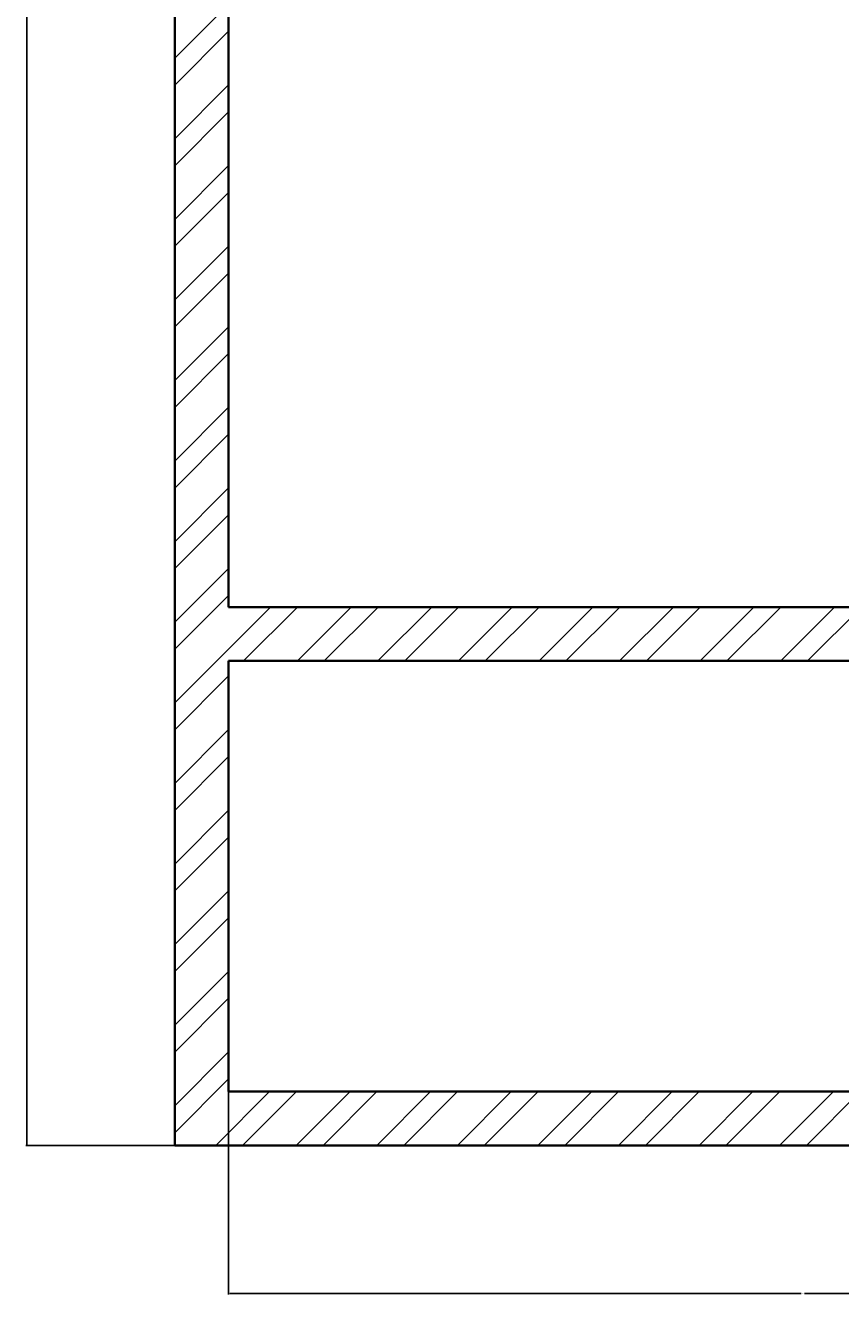
# Model space of a CAD drawing. Units: inches. Extents: x 2166 to 3588, y 1959 to 2628.
# Tile 3 of 13: x 3202 to 3339, y 1997 to 2209. Entities that reach past the tile are written whole.
import ezdxf

# ---------------------------------------------------------------- set-up
doc = ezdxf.new("R2010")
doc.units = ezdxf.units.IN
for name, color, linetype, lineweight in [('A-ANNO-DIMS', 2, 'Continuous', 18), ('A-WALL-PATT', 20, 'Continuous', 13), ('WALL', 40, 'Continuous', 35)]:
    doc.layers.add(name, color=color, linetype=linetype, lineweight=lineweight)
doc.styles.get("Standard").update_dxf_attribs({"font": 'arial.ttf'})
doc.dimstyles.get("Standard").update_dxf_attribs({"dimtxt": 0.18, "dimasz": 0.18, "dimexe": 0.18, "dimexo": 0.0625, "dimgap": 0.09, "dimtad": 0, "dimtih": 1, "dimtoh": 1, "dimdec": 4, "dimzin": 0, "dimdsep": 46, "dimtxsty": 'Standard', "dimcen": 0.09, "dimadec": 0, "dimazin": 0, "dimtfac": 1, "dimtdec": 4, "dimtofl": 0, "dimtmove": 0, "dimatfit": 3, "dimfxl": 1, "dimtolj": 1, "dimtzin": 0, "dimarcsym": 0})

# ---------------------------------------------------------------- blocks, each defined once
blk = doc.blocks.new('*D48')
at = {"layer": 'A-ANNO-DIMS', "color": 0, "lineweight": -2, "transparency": 16777216}
for p, q in [((3227.41, 2429.98), (3202.54, 2429.98)), ((3202.72, 2429.8), (3202.72, 2226.16)), ((3202.72, 2022.16), (3202.72, 2225.8)), ((3227.41, 2021.98), (3202.54, 2021.98))]:
    blk.add_line(p, q, dxfattribs=at)
at = {"layer": 'A-ANNO-DIMS', "color": 0, "transparency": 16777216}
for points in [[(3202.69, 2429.8), (3202.75, 2429.8), (3202.72, 2429.98)], [(3202.69, 2022.16), (3202.75, 2022.16), (3202.72, 2021.98)]]:
    blk.add_solid(points, dxfattribs=at)
at = {"layer": 'Defpoints', "color": 0, "transparency": 16777216}
for p in [(3202.72, 2429.98), (3227.47, 2429.98), (3227.47, 2021.98)]:
    blk.add_point(p, dxfattribs=at)
at = {"layer": 'A-ANNO-DIMS', "color": 0, "transparency": 16777216, "insert": (3202.72, 2225.98), "char_height": 0.18, "attachment_point": 5}
blk.add_mtext('\\A1;408', dxfattribs=at)
blk = doc.blocks.new('*D50')
at = {"layer": 'A-ANNO-DIMS', "color": 0, "lineweight": -2, "transparency": 16777216}
for p, q in [((3236.47, 2030.92), (3236.47, 1997.05)), ((3428.47, 2030.92), (3428.47, 1997.05)), ((3236.65, 1997.23), (3332.19, 1997.23)), ((3428.29, 1997.23), (3332.75, 1997.23))]:
    blk.add_line(p, q, dxfattribs=at)
at = {"layer": 'A-ANNO-DIMS', "color": 0, "transparency": 16777216}
for points in [[(3236.65, 1997.26), (3236.65, 1997.2), (3236.47, 1997.23)], [(3428.29, 1997.26), (3428.29, 1997.2), (3428.47, 1997.23)]]:
    blk.add_solid(points, dxfattribs=at)
at = {"layer": 'Defpoints', "color": 0, "transparency": 16777216}
for p in [(3236.47, 2030.98), (3428.47, 2030.98), (3428.47, 1997.23)]:
    blk.add_point(p, dxfattribs=at)
at = {"layer": 'A-ANNO-DIMS', "color": 0, "transparency": 16777216, "insert": (3332.47, 1997.23), "char_height": 0.18, "attachment_point": 5}
blk.add_mtext('\\A1;192', dxfattribs=at)

msp = doc.modelspace()

# ---------------------------------------------------------------- hatches: boundary and pattern name
at = {"layer": 'A-WALL-PATT'}
h = msp.add_hatch(dxfattribs=at)
h.set_pattern_fill('ANSI32', color=256)
h.paths.add_polyline_path([(3563.471, 2429.979), (3227.471, 2429.979), (3227.471, 2021.979), (3563.471, 2021.979)])
h.paths.add_polyline_path([(3236.471, 2420.979), (3554.471, 2420.979), (3554.471, 2111.979), (3236.471, 2111.979)], flags=16)
h.paths.add_polyline_path([(3236.471, 2102.979), (3554.471, 2102.979), (3554.471, 2030.979), (3236.471, 2030.979)], flags=16)
h.paths.add_polyline_path([(3518.471, 2085.283), (3518.471, 2067.979), (3458.471, 2067.979), (3458.471, 2085.283)], flags=0)
h.paths.add_polyline_path([(3434.656, 2082.283), (3442.194, 2082.283), (3442.194, 2087.514), (3434.656, 2087.514)], flags=8)
h.paths.add_polyline_path([(3522.671, 2094.512), (3521.752, 2052.984), (3545.541, 2052.457), (3546.46, 2093.986)], flags=8)

# ---------------------------------------------------------------- linework, layer by layer
at = {"layer": 'WALL'}
for p, q in [((3554.471, 2111.979), (3236.471, 2111.979)), ((3554.471, 2102.979), (3236.471, 2102.979))]:
    msp.add_line(p, q, dxfattribs=at)
msp.add_lwpolyline([(3227.471, 2429.979), (3563.471, 2429.979), (3563.471, 2021.979), (3227.471, 2021.979)], close=True, dxfattribs=at)
for points in [[(3236.471, 2111.979), (3236.471, 2420.979), (3554.471, 2420.979), (3554.471, 2111.979)], [(3554.471, 2102.979), (3554.471, 2030.979), (3236.471, 2030.979), (3236.471, 2102.979)]]:
    msp.add_lwpolyline(points, dxfattribs=at)

# ---------------------------------------------------------------- dimensions: what is measured, and where the dimension line sits
at = {"layer": 'A-ANNO-DIMS'}
dim = msp.add_linear_dim(base=(3202.721, 2429.979), p1=(3227.471, 2021.979), p2=(3227.471, 2429.979), angle=90, dimstyle='Standard', override={"dimdec": 0, "dimlfac": 1, "dimrnd": 0, "dimzin": 0, "dimdsep": 46, "dimlunit": 2}, dxfattribs=at)
dim.commit()
dim.dimension.update_dxf_attribs({"geometry": '*D48', "text_midpoint": (3202.721, 2225.979)})
dim = msp.add_linear_dim(base=(3428.471, 1997.229), p1=(3236.471, 2030.979), p2=(3428.471, 2030.979), dimstyle='Standard', override={"dimdec": 0, "dimlfac": 1, "dimrnd": 0, "dimzin": 0, "dimdsep": 46, "dimlunit": 2}, dxfattribs=at)
dim.commit()
dim.dimension.update_dxf_attribs({"geometry": '*D50', "text_midpoint": (3332.471, 1997.229)})

doc.saveas('drawing.dxf')
